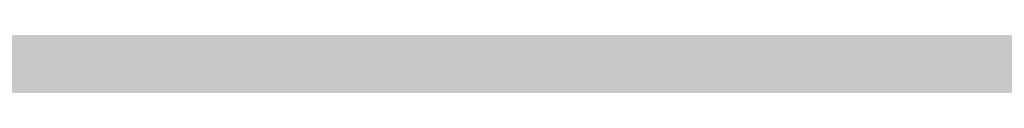
# Model space of a CAD drawing. Units: millimetres. Extents: x 0 to 2267, y 0 to 1823.
# Tile 54 of 256: x 1596.855 to 1600.369, y 1227.02 to 1227.171. Entities that reach past the tile are written whole.
import ezdxf

# ---------------------------------------------------------------- set-up
doc = ezdxf.new("R2010")
doc.units = ezdxf.units.MM
doc.header["$MEASUREMENT"] = 0
doc.layers.add('M-HATC', color=252, linetype='Continuous', lineweight=18)

msp = doc.modelspace()

# ---------------------------------------------------------------- hatches: boundary and pattern name
at = {"layer": 'M-HATC'}
h = msp.add_hatch(color=256, dxfattribs=at)
h.dxf.hatch_style = 1
h.paths.add_polyline_path([(2055.771, 1603.062), (1381.0868, 1603.062), (1381.0868, 1598.062), (2055.771, 1598.062)])
h.paths.add_polyline_path([(2055.771, 1598.062), (1381.0868, 1598.062), (1381.0868, 1593.062), (2055.771, 1593.062)])
h.paths.add_polyline_path([(2051.3074, 1536.7609), (1385.5504, 1536.7609), (1385.5504, 1526.7609), (1387.5504, 1526.7609), (1388.5366, 1525.0528), (1385.3319, 1521.2335), (1385.3319, 1521.2226), (2050.2542, 1522.7491), (2048.3212, 1525.0528), (2049.3074, 1526.7609), (2051.3074, 1526.7609)])
edge = h.paths.add_edge_path()
edge.add_arc((1847.5345, 1379.1492), 135, 222.603061, 222.890851, ccw=False)
edge.add_line((1748.1663, 1287.7656), (1683.0921, 1287.7656))
edge.add_arc((1583.7239, 1379.1492), 135, 317.109149, 317.396939, ccw=False)
edge.add_arc((1678.9686, 1290.6707), 5, 222.8909, 317.1091, ccw=False)
edge.add_arc((1774.2133, 1379.1492), 135, 222.603061, 222.890851, ccw=False)
edge.add_line((1674.8451, 1287.7656), (1609.7709, 1287.7656))
edge.add_arc((1510.4027, 1379.1492), 135, 317.109149, 317.396939, ccw=False)
edge.add_arc((1605.6474, 1290.6707), 5, 222.8909, 317.1091, ccw=False)
edge.add_arc((1700.8921, 1379.1492), 135, 222.603061, 222.890851, ccw=False)
edge.add_line((1601.5239, 1287.7656), (1536.4497, 1287.7656))
edge.add_arc((1437.0815, 1379.1492), 135, 317.109149, 317.396939, ccw=False)
edge.add_arc((1532.3262, 1290.6707), 5, 222.8909, 317.1091, ccw=False)
edge.add_arc((1627.5709, 1379.1492), 135, 222.603061, 222.890851, ccw=False)
edge.add_line((1528.2027, 1287.7656), (1505.9289, 1287.7656))
edge.add_spline(control_points=[(1505.9289, 1287.7656), (1504.2622, 1287.7656), (1504.2622, 1282.7656), (1505.9289, 1282.7656)], knot_values=[0, 0, 0, 0, 5, 5, 5, 5], degree=3, periodic=0)
edge.add_line((1505.9289, 1282.7656), (1930.9289, 1282.7656))
edge.add_spline(control_points=[(1930.9289, 1282.7656), (1932.5956, 1282.7656), (1932.5956, 1287.7656), (1930.9289, 1287.7656)], knot_values=[0, 0, 0, 0, 5, 5, 5, 5], degree=3, periodic=0)
edge.add_line((1930.9289, 1287.7656), (1903.0557, 1287.7656))
edge.add_arc((1803.6875, 1379.1492), 135, 317.109149, 317.396939, ccw=False)
edge.add_arc((1898.9322, 1290.6707), 5, 222.8909, 317.1091, ccw=False)
edge.add_arc((1994.1769, 1379.1492), 135, 222.603061, 222.890851, ccw=False)
edge.add_line((1894.8087, 1287.7656), (1829.7345, 1287.7656))
edge.add_arc((1730.3663, 1379.1492), 135, 317.109149, 317.396939, ccw=False)
edge.add_arc((1825.611, 1290.6707), 5, 222.8909, 317.1091, ccw=False)
edge.add_arc((1920.8557, 1379.1492), 135, 222.603061, 222.890851, ccw=False)
edge.add_line((1821.4875, 1287.7656), (1756.4133, 1287.7656))
edge.add_arc((1657.0451, 1379.1492), 135, 317.109149, 317.396939, ccw=False)
edge.add_arc((1752.2898, 1290.6707), 5, 222.8909, 317.1091, ccw=False)
edge = h.paths.add_edge_path()
edge.add_spline(control_points=[(1843.4289, 1227.2475), (1845.0956, 1227.2475), (1845.0956, 1232.2475), (1843.4289, 1232.2475)], knot_values=[0, 0, 0, 0, 5, 5, 5, 5], degree=3, periodic=0)
edge.add_line((1843.4289, 1232.2475), (1593.4289, 1232.2475))
edge.add_spline(control_points=[(1593.4289, 1232.2475), (1591.7622, 1232.2475), (1591.7622, 1227.2475), (1593.4289, 1227.2475)], knot_values=[0, 0, 0, 0, 5, 5, 5, 5], degree=3, periodic=0)
edge.add_line((1593.4289, 1227.2475), (1843.4289, 1227.2475))
h.paths.add_polyline_path([(1905.9289, 1127.4171), (1530.9289, 1127.4171, 0.414214), (1520.9289, 1117.4171), (1530.9289, 1117.4171), (1915.9289, 1117.4171, 0.414214)])
edge = h.paths.add_edge_path()
edge.add_arc((1397.0858, 1498.4078), 12.7299, 90.78215, 190.87871, ccw=False)
edge.add_line((1396.912, 1511.1365), (1428.0097, 1511.3488))
edge.add_line((1428.0097, 1511.3488), (1433.0097, 1511.3488))
edge.add_line((1433.0097, 1511.3488), (1434.439, 1511.3488))
edge.add_arc((1419.474, 1498.0804), 20, 41.561, 74.08211)
edge.add_line((1424.9592, 1517.3135), (1399.9351, 1517.2561))
edge.add_spline(control_points=[(1399.9307, 1517.2561), (1399.884, 1517.2131), (1399.8328, 1517.1689), (1399.7774, 1517.1236)], knot_values=[11.567499, 11.567499, 11.567499, 11.567499, 11.814249, 11.814249, 11.814249, 11.814249], degree=3, periodic=0)
edge.add_spline(control_points=[(1399.6328, 1517.0099), (1399.5831, 1516.9721), (1399.5307, 1516.9338), (1399.4759, 1516.8947)], knot_values=[11.167718, 11.167718, 11.167718, 11.167718, 11.365188, 11.365188, 11.365188, 11.365188], degree=3, periodic=0)
edge.add_spline(control_points=[(1399.3398, 1516.8001), (1399.1514, 1516.6719), (1398.9384, 1516.5377), (1398.704, 1516.3994)], knot_values=[10.376405, 10.376405, 10.376405, 10.376405, 11.00994, 11.00994, 11.00994, 11.00994], degree=3, periodic=0)
edge.add_spline(control_points=[(1398.6572, 1516.3719), (1398.5789, 1516.326), (1398.4983, 1516.2797), (1398.4155, 1516.2331)], knot_values=[10.125175, 10.125175, 10.125175, 10.125175, 10.334406, 10.334406, 10.334406, 10.334406], degree=3, periodic=0)
edge.add_spline(control_points=[(1398.2642, 1516.1487), (1398.196, 1516.1111), (1398.1263, 1516.0732), (1398.0555, 1516.0351)], knot_values=[9.832246, 9.832246, 9.832246, 9.832246, 9.999658, 9.999658, 9.999658, 9.999658], degree=3, periodic=0)
edge.add_spline(control_points=[(1397.9987, 1516.0048), (1397.7312, 1515.8621), (1397.446, 1515.7171), (1397.1466, 1515.5714)], knot_values=[9.161808, 9.161808, 9.161808, 9.161808, 9.787769, 9.787769, 9.787769, 9.787769], degree=3, periodic=0)
edge.add_spline(control_points=[(1397.1466, 1515.5714), (1396.8418, 1515.423), (1396.5222, 1515.274), (1396.1914, 1515.1262)], knot_values=[8.524455, 8.524455, 8.524455, 8.524455, 9.161808, 9.161808, 9.161808, 9.161808], degree=3, periodic=0)
edge.add_spline(control_points=[(1396.0777, 1515.0756), (1395.9854, 1515.0348), (1395.8922, 1514.994), (1395.7983, 1514.9534)], knot_values=[8.275193, 8.275193, 8.275193, 8.275193, 8.451726, 8.451726, 8.451726, 8.451726], degree=3, periodic=0)
edge.add_spline(control_points=[(1395.6018, 1514.8691), (1395.4997, 1514.8257), (1395.3968, 1514.7824), (1395.2932, 1514.7394)], knot_values=[7.962917, 7.962917, 7.962917, 7.962917, 8.152764, 8.152764, 8.152764, 8.152764], degree=3, periodic=0)
edge.add_spline(control_points=[(1395.2116, 1514.7057), (1394.8278, 1514.5475), (1394.4345, 1514.3929), (1394.0364, 1514.2442)], knot_values=[7.21254, 7.21254, 7.21254, 7.21254, 7.913148, 7.913148, 7.913148, 7.913148], degree=3, periodic=0)
edge.add_spline(control_points=[(1394.0364, 1514.2442), (1393.7076, 1514.1214), (1393.3754, 1514.0027), (1393.0427, 1513.8895)], knot_values=[6.633733, 6.633733, 6.633733, 6.633733, 7.21254, 7.21254, 7.21254, 7.21254], degree=3, periodic=0)
edge.add_spline(control_points=[(1392.8214, 1513.815), (1392.7198, 1513.7812), (1392.6181, 1513.7479), (1392.5166, 1513.7152)], knot_values=[6.328796, 6.328796, 6.328796, 6.328796, 6.505493, 6.505493, 6.505493, 6.505493], degree=3, periodic=0)
edge.add_spline(control_points=[(1392.5166, 1513.7152), (1392.3187, 1513.6515), (1392.1212, 1513.59), (1391.9244, 1513.531)], knot_values=[5.984605, 5.984605, 5.984605, 5.984605, 6.328796, 6.328796, 6.328796, 6.328796], degree=3, periodic=0)
edge.add_spline(control_points=[(1391.7915, 1513.4915), (1391.3122, 1513.3501), (1390.8384, 1513.2239), (1390.3784, 1513.1171)], knot_values=[5.066697, 5.066697, 5.066697, 5.066697, 5.907055, 5.907055, 5.907055, 5.907055], degree=3, periodic=0)
edge.add_spline(control_points=[(1390.3784, 1513.1171), (1390.1797, 1513.071), (1389.9836, 1513.0284), (1389.7907, 1512.9899)], knot_values=[4.70367, 4.70367, 4.70367, 4.70367, 5.066695, 5.066695, 5.066695, 5.066695], degree=3, periodic=0)
edge.add_spline(control_points=[(1389.422, 1512.9204), (1389.2459, 1512.8892), (1389.0729, 1512.8617), (1388.9036, 1512.8381)], knot_values=[4.130571, 4.130571, 4.130571, 4.130571, 4.469816, 4.469816, 4.469816, 4.469816], degree=3, periodic=0)
edge.add_spline(control_points=[(1388.9036, 1512.8381), (1388.591, 1512.7946), (1388.2911, 1512.7644), (1388.0071, 1512.7494)], knot_values=[3.504031, 3.504031, 3.504031, 3.504031, 4.130571, 4.130571, 4.130571, 4.130571], degree=3, periodic=0)
edge.add_spline(control_points=[(1387.9356, 1512.7459), (1387.8538, 1512.7423), (1387.7733, 1512.74), (1387.6944, 1512.739)], knot_values=[3.268866, 3.268866, 3.268866, 3.268866, 3.451164, 3.451164, 3.451164, 3.451164], degree=3, periodic=0)
edge.add_spline(control_points=[(1387.3351, 1512.7443), (1387.2076, 1512.7499), (1387.0847, 1512.7597), (1386.967, 1512.7739)], knot_values=[2.670686, 2.670686, 2.670686, 2.670686, 2.984, 2.984, 2.984, 2.984], degree=3, periodic=0)
edge.add_spline(control_points=[(1386.8327, 1512.7922), (1386.8209, 1512.7941), (1386.8092, 1512.7959), (1386.7975, 1512.7979)], knot_values=[2.516981, 2.516981, 2.516981, 2.516981, 2.549528, 2.549528, 2.549528, 2.549528], degree=3, periodic=0)
edge.add_spline(control_points=[(1386.4526, 1512.8735), (1386.4257, 1512.881), (1386.3993, 1512.889), (1386.3733, 1512.8972)], knot_values=[2.095869, 2.095869, 2.095869, 2.095869, 2.17941, 2.17941, 2.17941, 2.17941], degree=3, periodic=0)
edge.add_spline(control_points=[(1386.0691, 1513.0189), (1386.0634, 1513.0217), (1386.0577, 1513.0246), (1386.052, 1513.0275)], knot_values=[1.72453, 1.72453, 1.72453, 1.72453, 1.745933, 1.745933, 1.745933, 1.745933], degree=3, periodic=0)
edge.add_arc((1399.474, 1498.0804), 20, 131.82432, 180)
edge.add_arc((1630.3336, 1505.5484), 250.9708, 181.705176, 236.427975)
edge.add_arc((1605.3399, 1483.3044), 218.7822, 238.660829, 243.34961)
edge.add_arc((1647.0911, 1510.3592), 262.8986, 183.129836, 237.853442, ccw=False)
h.paths.add_polyline_path([(1406.5369, 1391.9644, 0.149382), (1491.5506, 1296.4418, -0.129517)], flags=17)
edge = h.paths.add_edge_path()
edge.add_arc((2037.3838, 1498.0804), 20, 0, 48.26587)
edge.add_spline(control_points=[(2050.6973, 1513.0052), (2050.6512, 1512.9847), (2050.6034, 1512.9655), (2050.5539, 1512.9477)], knot_values=[1.835652, 1.835652, 1.835652, 1.835652, 2.000781, 2.000781, 2.000781, 2.000781], degree=3, periodic=0)
edge.add_spline(control_points=[(2050.4616, 1512.9166), (2050.479, 1512.9221), (2050.4963, 1512.9277), (2050.5133, 1512.9335)], knot_values=[2.045477, 2.045477, 2.045477, 2.045477, 2.101389, 2.101389, 2.101389, 2.101389], degree=3, periodic=0)
edge.add_spline(control_points=[(2050.129, 1512.8342), (2050.1984, 1512.8473), (2050.2657, 1512.8623), (2050.3308, 1512.8792)], knot_values=[2.237629, 2.237629, 2.237629, 2.237629, 2.435841, 2.435841, 2.435841, 2.435841], degree=3, periodic=0)
edge.add_spline(control_points=[(2050.0946, 1512.8278), (2050.1061, 1512.8299), (2050.1176, 1512.832), (2050.129, 1512.8342)], knot_values=[2.435841, 2.435841, 2.435841, 2.435841, 2.468321, 2.468321, 2.468321, 2.468321], degree=3, periodic=0)
edge.add_spline(control_points=[(2049.7843, 1512.7851), (2049.8552, 1512.7922), (2049.9243, 1512.8008), (2049.9917, 1512.8109)], knot_values=[2.563852, 2.563852, 2.563852, 2.563852, 2.748541, 2.748541, 2.748541, 2.748541], degree=3, periodic=0)
edge.add_spline(control_points=[(2049.4052, 1512.7617), (2049.5364, 1512.7653), (2049.6629, 1512.773), (2049.7843, 1512.7851)], knot_values=[2.748541, 2.748541, 2.748541, 2.748541, 3.064882, 3.064882, 3.064882, 3.064882], degree=3, periodic=0)
edge.add_spline(control_points=[(2049.1698, 1512.7597), (2049.2336, 1512.7591), (2049.2965, 1512.7594), (2049.3584, 1512.7606)], knot_values=[3.102309, 3.102309, 3.102309, 3.102309, 3.2503, 3.2503, 3.2503, 3.2503], degree=3, periodic=0)
edge.add_spline(control_points=[(2048.8573, 1512.7691), (2048.9638, 1512.7638), (2049.068, 1512.7606), (2049.1698, 1512.7597)], knot_values=[3.2503, 3.2503, 3.2503, 3.2503, 3.486069, 3.486069, 3.486069, 3.486069], degree=3, periodic=0)
edge.add_spline(control_points=[(2048.6924, 1512.7789), (2048.3729, 1512.8009), (2048.0345, 1512.8411), (2047.6817, 1512.897)], knot_values=[3.606429, 3.606429, 3.606429, 3.606429, 4.2989, 4.2989, 4.2989, 4.2989], degree=3, periodic=0)
edge.add_spline(control_points=[(2047.6817, 1512.897), (2047.5458, 1512.9185), (2047.4077, 1512.9424), (2047.2678, 1512.9685)], knot_values=[4.2989, 4.2989, 4.2989, 4.2989, 4.565769, 4.565769, 4.565769, 4.565769], degree=3, periodic=0)
edge.add_spline(control_points=[(2047.2678, 1512.9685), (2047.1449, 1512.9914), (2047.0207, 1513.016), (2046.8951, 1513.0422)], knot_values=[4.565769, 4.565769, 4.565769, 4.565769, 4.799971, 4.799971, 4.799971, 4.799971], degree=3, periodic=0)
edge.add_spline(control_points=[(2046.8951, 1513.0422), (2046.5286, 1513.1188), (2046.1513, 1513.209), (2045.7676, 1513.3107)], knot_values=[4.799971, 4.799971, 4.799971, 4.799971, 5.483718, 5.483718, 5.483718, 5.483718], degree=3, periodic=0)
edge.add_spline(control_points=[(2045.7676, 1513.3107), (2045.3724, 1513.4154), (2044.9704, 1513.5322), (2044.5662, 1513.6588)], knot_values=[5.483718, 5.483718, 5.483718, 5.483718, 6.187866, 6.187866, 6.187866, 6.187866], degree=3, periodic=0)
edge.add_spline(control_points=[(2044.5662, 1513.6588), (2044.4149, 1513.7061), (2044.2633, 1513.7549), (2044.1116, 1513.8048)], knot_values=[6.187866, 6.187866, 6.187866, 6.187866, 6.451551, 6.451551, 6.451551, 6.451551], degree=3, periodic=0)
edge.add_spline(control_points=[(2044.1116, 1513.8048), (2043.9967, 1513.8427), (2043.8817, 1513.8813), (2043.7668, 1513.9205)], knot_values=[6.451551, 6.451551, 6.451551, 6.451551, 6.651434, 6.651434, 6.651434, 6.651434], degree=3, periodic=0)
edge.add_spline(control_points=[(2043.7668, 1513.9205), (2043.3716, 1514.0554), (2042.9774, 1514.1979), (2042.5886, 1514.3458)], knot_values=[6.651434, 6.651434, 6.651434, 6.651434, 7.338879, 7.338879, 7.338879, 7.338879], degree=3, periodic=0)
edge.add_spline(control_points=[(2042.5886, 1514.3458), (2042.1643, 1514.5071), (2041.7465, 1514.6749), (2041.3409, 1514.846)], knot_values=[7.338879, 7.338879, 7.338879, 7.338879, 8.089209, 8.089209, 8.089209, 8.089209], degree=3, periodic=0)
edge.add_spline(control_points=[(2041.3409, 1514.846), (2041.1028, 1514.9465), (2040.869, 1515.0481), (2040.6405, 1515.1502)], knot_values=[8.089209, 8.089209, 8.089209, 8.089209, 8.529587, 8.529587, 8.529587, 8.529587], degree=3, periodic=0)
edge.add_spline(control_points=[(2040.51, 1515.2089), (2040.0824, 1515.4022), (2039.6747, 1515.5971), (2039.295, 1515.7894)], knot_values=[8.613818, 8.613818, 8.613818, 8.613818, 9.44571, 9.44571, 9.44571, 9.44571], degree=3, periodic=0)
edge.add_spline(control_points=[(2039.295, 1515.7894), (2039.0618, 1515.9075), (2038.8391, 1516.0246), (2038.6288, 1516.1398)], knot_values=[9.44571, 9.44571, 9.44571, 9.44571, 9.956404, 9.956404, 9.956404, 9.956404], degree=3, periodic=0)
edge.add_spline(control_points=[(2038.6288, 1516.1398), (2038.5187, 1516.2001), (2038.4121, 1516.2598), (2038.309, 1516.3189)], knot_values=[9.956404, 9.956404, 9.956404, 9.956404, 10.223542, 10.223542, 10.223542, 10.223542], degree=3, periodic=0)
edge.add_spline(control_points=[(2038.309, 1516.3189), (2038.2138, 1516.3735), (2038.1216, 1516.4276), (2038.0328, 1516.481)], knot_values=[10.223542, 10.223542, 10.223542, 10.223542, 10.47051, 10.47051, 10.47051, 10.47051], degree=3, periodic=0)
edge.add_spline(control_points=[(2038.0328, 1516.481), (2037.7855, 1516.6296), (2037.5639, 1516.773), (2037.3722, 1516.909)], knot_values=[10.47051, 10.47051, 10.47051, 10.47051, 11.15767, 11.15767, 11.15767, 11.15767], degree=3, periodic=0)
edge.add_spline(control_points=[(2037.3722, 1516.909), (2037.2789, 1516.9752), (2037.1927, 1517.0396), (2037.1142, 1517.102)], knot_values=[11.15767, 11.15767, 11.15767, 11.15767, 11.49227, 11.49227, 11.49227, 11.49227], degree=3, periodic=0)
edge.add_spline(control_points=[(2036.8564, 1517.3259), (2036.9148, 1517.2692), (2036.9814, 1517.2103), (2037.0557, 1517.1492)], knot_values=[11.577341, 11.577341, 11.577341, 11.577341, 11.91035, 11.91035, 11.91035, 11.91035], degree=3, periodic=0)
edge.add_spline(control_points=[(2036.8074, 1517.3748), (2036.823, 1517.3587), (2036.8393, 1517.3424), (2036.8564, 1517.3259)], knot_values=[11.91035, 11.91035, 11.91035, 11.91035, 12.007402, 12.007402, 12.007402, 12.007402], degree=3, periodic=0)
edge.add_spline(control_points=[(2036.7017, 1517.494), (2036.7104, 1517.483), (2036.7196, 1517.4719), (2036.7291, 1517.4606)], knot_values=[12.184155, 12.184155, 12.184155, 12.184155, 12.255409, 12.255409, 12.255409, 12.255409], degree=3, periodic=0)
edge.add_spline(control_points=[(2036.6159, 1517.6205), (2036.62, 1517.613), (2036.6243, 1517.6055), (2036.6289, 1517.5979)], knot_values=[12.487913, 12.487913, 12.487913, 12.487913, 12.541035, 12.541035, 12.541035, 12.541035], degree=3, periodic=0)
edge.add_spline(control_points=[(2036.5635, 1517.786), (2036.5637, 1517.7794), (2036.5642, 1517.7726), (2036.565, 1517.7658)], knot_values=[12.911761, 12.911761, 12.911761, 12.911761, 12.968286, 12.968286, 12.968286, 12.968286], degree=3, periodic=0)
edge.add_spline(control_points=[(2036.6166, 1517.9304), (2036.6125, 1517.9259), (2036.6086, 1517.9212), (2036.6049, 1517.9165)], knot_values=[13.382527, 13.382527, 13.382527, 13.382527, 13.433791, 13.433791, 13.433791, 13.433791], degree=3, periodic=0)
edge.add_spline(control_points=[(2036.749, 1518.017), (2036.7361, 1518.0116), (2036.7239, 1518.006), (2036.7124, 1518.0002)], knot_values=[13.726299, 13.726299, 13.726299, 13.726299, 13.809928, 13.809928, 13.809928, 13.809928], degree=3, periodic=0)
edge.add_spline(control_points=[(2036.8604, 1518.0528), (2036.8386, 1518.0474), (2036.8181, 1518.0416), (2036.7988, 1518.0353)], knot_values=[13.910887, 13.910887, 13.910887, 13.910887, 14.02153, 14.02153, 14.02153, 14.02153], degree=3, periodic=0)
edge.add_line((2036.9639, 1518.0804), (2032.3838, 1518.0804))
edge.add_line((2032.3838, 1518.0804), (2027.3838, 1518.0804))
edge.add_line((2027.3838, 1518.0804), (2022.3838, 1518.0804))
edge.add_line((2022.3838, 1518.0804), (2017.3838, 1518.0804))
edge.add_arc((2017.3838, 1498.0804), 20, 90, 138.439)
edge.add_line((2002.4188, 1511.3488), (2003.8481, 1511.3488))
edge.add_line((2003.8481, 1511.3488), (2008.8481, 1511.3488))
edge.add_line((2008.8481, 1511.3488), (2039.772, 1511.1377))
edge.add_arc((2039.772, 1498.4078), 12.7299, -10.87871, 90, ccw=False)
edge.add_arc((1789.7668, 1510.3592), 262.8986, 302.146558, 356.870164, ccw=False)
edge.add_arc((1831.5179, 1483.3044), 218.7822, 296.65039, 301.339171)
edge.add_arc((1806.5242, 1505.5484), 250.9708, 303.572025, 358.294824)
h.paths.add_polyline_path([(2030.321, 1391.9644, -0.129517), (1945.3072, 1296.4418, 0.149382)], flags=17)
edge = h.paths.add_edge_path()
edge.add_spline(control_points=[(2037.2464, 1518.0821), (2037.2898, 1518.081), (2037.3355, 1518.0804), (2037.3838, 1518.0804)], knot_values=[0.000012, 0.000012, 0.000012, 0.000012, 0.144754, 0.144754, 0.144754, 0.144754], degree=3, periodic=0)
edge.add_line((2037.3357, 1518.0804), (2037.0096, 1518.0804))
edge.add_spline(control_points=[(2037.0096, 1518.0804), (2036.9822, 1518.0768), (2036.956, 1518.0727), (2036.9312, 1518.0681)], knot_values=[14.13465, 14.13465, 14.13465, 14.13465, 14.247197, 14.247197, 14.247197, 14.247197], degree=3, periodic=0)
edge.add_spline(control_points=[(2036.9312, 1518.0681), (2036.9276, 1518.0674), (2036.9241, 1518.0667), (2036.9205, 1518.0661)], knot_values=[14.118315, 14.118315, 14.118315, 14.118315, 14.13465, 14.13465, 14.13465, 14.13465], degree=3, periodic=0)
edge.add_spline(control_points=[(2036.9205, 1518.0661), (2036.9118, 1518.0644), (2036.9032, 1518.0626), (2036.8948, 1518.0608)], knot_values=[14.078086, 14.078086, 14.078086, 14.078086, 14.118315, 14.118315, 14.118315, 14.118315], degree=3, periodic=0)
edge.add_spline(control_points=[(2036.8948, 1518.0608), (2036.883, 1518.0583), (2036.8716, 1518.0556), (2036.8604, 1518.0528)], knot_values=[14.02153, 14.02153, 14.02153, 14.02153, 14.078086, 14.078086, 14.078086, 14.078086], degree=3, periodic=0)
edge.add_spline(control_points=[(2036.8604, 1518.0528), (2036.8386, 1518.0474), (2036.8181, 1518.0416), (2036.7988, 1518.0353)], knot_values=[13.910887, 13.910887, 13.910887, 13.910887, 14.02153, 14.02153, 14.02153, 14.02153], degree=3, periodic=0)
edge.add_spline(control_points=[(2036.7988, 1518.0353), (2036.7981, 1518.035), (2036.7974, 1518.0348), (2036.7967, 1518.0346)], knot_values=[13.906906, 13.906906, 13.906906, 13.906906, 13.910887, 13.910887, 13.910887, 13.910887], degree=3, periodic=0)
edge.add_spline(control_points=[(2036.7967, 1518.0346), (2036.7882, 1518.0318), (2036.7799, 1518.0289), (2036.7719, 1518.0259)], knot_values=[13.857826, 13.857826, 13.857826, 13.857826, 13.906906, 13.906906, 13.906906, 13.906906], degree=3, periodic=0)
edge.add_spline(control_points=[(2036.7719, 1518.0259), (2036.764, 1518.023), (2036.7564, 1518.02), (2036.749, 1518.017)], knot_values=[13.809928, 13.809928, 13.809928, 13.809928, 13.857826, 13.857826, 13.857826, 13.857826], degree=3, periodic=0)
edge.add_spline(control_points=[(2036.749, 1518.017), (2036.7361, 1518.0116), (2036.7239, 1518.006), (2036.7124, 1518.0002)], knot_values=[13.726299, 13.726299, 13.726299, 13.726299, 13.809928, 13.809928, 13.809928, 13.809928], degree=3, periodic=0)
edge.add_spline(control_points=[(2036.7124, 1518.0002), (2036.7121, 1518), (2036.7118, 1517.9999), (2036.7115, 1517.9997)], knot_values=[13.723993, 13.723993, 13.723993, 13.723993, 13.726299, 13.726299, 13.726299, 13.726299], degree=3, periodic=0)
edge.add_spline(control_points=[(2036.7115, 1517.9997), (2036.7063, 1517.9971), (2036.7013, 1517.9944), (2036.6965, 1517.9917)], knot_values=[13.686536, 13.686536, 13.686536, 13.686536, 13.723993, 13.723993, 13.723993, 13.723993], degree=3, periodic=0)
edge.add_spline(control_points=[(2036.6965, 1517.9917), (2036.6919, 1517.9891), (2036.6874, 1517.9865), (2036.6831, 1517.9839)], knot_values=[13.651251, 13.651251, 13.651251, 13.651251, 13.686536, 13.686536, 13.686536, 13.686536], degree=3, periodic=0)
edge.add_spline(control_points=[(2036.6831, 1517.9839), (2036.6764, 1517.9798), (2036.67, 1517.9757), (2036.6639, 1517.9714)], knot_values=[13.596804, 13.596804, 13.596804, 13.596804, 13.651251, 13.651251, 13.651251, 13.651251], degree=3, periodic=0)
edge.add_spline(control_points=[(2036.6639, 1517.9714), (2036.6636, 1517.9712), (2036.6633, 1517.9709), (2036.6629, 1517.9707)], knot_values=[13.593956, 13.593956, 13.593956, 13.593956, 13.596804, 13.596804, 13.596804, 13.596804], degree=3, periodic=0)
edge.add_spline(control_points=[(2036.6629, 1517.9707), (2036.6603, 1517.9689), (2036.6577, 1517.967), (2036.6552, 1517.9651)], knot_values=[13.570322, 13.570322, 13.570322, 13.570322, 13.593956, 13.593956, 13.593956, 13.593956], degree=3, periodic=0)
edge.add_spline(control_points=[(2036.6552, 1517.9651), (2036.6525, 1517.9631), (2036.6499, 1517.9611), (2036.6474, 1517.9591)], knot_values=[13.545477, 13.545477, 13.545477, 13.545477, 13.570322, 13.570322, 13.570322, 13.570322], degree=3, periodic=0)
edge.add_spline(control_points=[(2036.6474, 1517.9591), (2036.6472, 1517.9589), (2036.6471, 1517.9588), (2036.6469, 1517.9587)], knot_values=[13.543931, 13.543931, 13.543931, 13.543931, 13.545477, 13.545477, 13.545477, 13.545477], degree=3, periodic=0)
edge.add_spline(control_points=[(2036.6469, 1517.9587), (2036.6412, 1517.9541), (2036.6358, 1517.9494), (2036.6307, 1517.9447)], knot_values=[13.488237, 13.488237, 13.488237, 13.488237, 13.543931, 13.543931, 13.543931, 13.543931], degree=3, periodic=0)
edge.add_spline(control_points=[(2036.6307, 1517.9447), (2036.6282, 1517.9423), (2036.6257, 1517.9399), (2036.6233, 1517.9374)], knot_values=[13.460307, 13.460307, 13.460307, 13.460307, 13.488237, 13.488237, 13.488237, 13.488237], degree=3, periodic=0)
edge.add_spline(control_points=[(2036.6233, 1517.9374), (2036.6215, 1517.9356), (2036.6198, 1517.9338), (2036.6181, 1517.932)], knot_values=[13.439712, 13.439712, 13.439712, 13.439712, 13.460307, 13.460307, 13.460307, 13.460307], degree=3, periodic=0)
edge.add_spline(control_points=[(2036.6181, 1517.932), (2036.6176, 1517.9315), (2036.6171, 1517.9309), (2036.6166, 1517.9304)], knot_values=[13.433791, 13.433791, 13.433791, 13.433791, 13.439712, 13.439712, 13.439712, 13.439712], degree=3, periodic=0)
edge.add_spline(control_points=[(2036.6166, 1517.9304), (2036.6125, 1517.9259), (2036.6086, 1517.9212), (2036.6049, 1517.9165)], knot_values=[13.382527, 13.382527, 13.382527, 13.382527, 13.433791, 13.433791, 13.433791, 13.433791], degree=3, periodic=0)
edge.add_spline(control_points=[(2036.6049, 1517.9165), (2036.6026, 1517.9135), (2036.6004, 1517.9104), (2036.5982, 1517.9074)], knot_values=[13.350017, 13.350017, 13.350017, 13.350017, 13.382527, 13.382527, 13.382527, 13.382527], degree=3, periodic=0)
edge.add_spline(control_points=[(2036.5982, 1517.9074), (2036.5972, 1517.9059), (2036.5962, 1517.9043), (2036.5952, 1517.9028)], knot_values=[13.333922, 13.333922, 13.333922, 13.333922, 13.350017, 13.350017, 13.350017, 13.350017], degree=3, periodic=0)
edge.add_spline(control_points=[(2036.5952, 1517.9028), (2036.5945, 1517.9018), (2036.5939, 1517.9009), (2036.5933, 1517.8999)], knot_values=[13.323828, 13.323828, 13.323828, 13.323828, 13.333922, 13.333922, 13.333922, 13.333922], degree=3, periodic=0)
edge.add_spline(control_points=[(2036.5933, 1517.8999), (2036.5905, 1517.8955), (2036.5879, 1517.8909), (2036.5855, 1517.8864)], knot_values=[13.277545, 13.277545, 13.277545, 13.277545, 13.323828, 13.323828, 13.323828, 13.323828], degree=3, periodic=0)
edge.add_spline(control_points=[(2036.5855, 1517.8864), (2036.5836, 1517.8827), (2036.5817, 1517.8789), (2036.5801, 1517.8751)], knot_values=[13.240119, 13.240119, 13.240119, 13.240119, 13.277545, 13.277545, 13.277545, 13.277545], degree=3, periodic=0)
edge.add_spline(control_points=[(2036.5801, 1517.8751), (2036.5795, 1517.8739), (2036.579, 1517.8727), (2036.5785, 1517.8715)], knot_values=[13.228211, 13.228211, 13.228211, 13.228211, 13.240119, 13.240119, 13.240119, 13.240119], degree=3, periodic=0)
edge.add_spline(control_points=[(2036.5785, 1517.8715), (2036.578, 1517.8702), (2036.5774, 1517.869), (2036.5769, 1517.8677)], knot_values=[13.215717, 13.215717, 13.215717, 13.215717, 13.228211, 13.228211, 13.228211, 13.228211], degree=3, periodic=0)
edge.add_spline(control_points=[(2036.5769, 1517.8677), (2036.5755, 1517.864), (2036.5741, 1517.8603), (2036.5729, 1517.8565)], knot_values=[13.179847, 13.179847, 13.179847, 13.179847, 13.215717, 13.215717, 13.215717, 13.215717], degree=3, periodic=0)
edge.add_spline(control_points=[(2036.5729, 1517.8565), (2036.5713, 1517.8515), (2036.5699, 1517.8464), (2036.5687, 1517.8413)], knot_values=[13.132017, 13.132017, 13.132017, 13.132017, 13.179847, 13.179847, 13.179847, 13.179847], degree=3, periodic=0)
edge.add_spline(control_points=[(2036.5687, 1517.8413), (2036.5684, 1517.8402), (2036.5682, 1517.8392), (2036.568, 1517.8382)], knot_values=[13.122482, 13.122482, 13.122482, 13.122482, 13.132017, 13.132017, 13.132017, 13.132017], degree=3, periodic=0)
edge.add_spline(control_points=[(2036.568, 1517.8382), (2036.5676, 1517.8363), (2036.5672, 1517.8345), (2036.5669, 1517.8327)], knot_values=[13.105592, 13.105592, 13.105592, 13.105592, 13.122482, 13.122482, 13.122482, 13.122482], degree=3, periodic=0)
edge.add_spline(control_points=[(2036.5669, 1517.8327), (2036.5662, 1517.8292), (2036.5657, 1517.8257), (2036.5652, 1517.8222)], knot_values=[13.074063, 13.074063, 13.074063, 13.074063, 13.105592, 13.105592, 13.105592, 13.105592], degree=3, periodic=0)
edge.add_spline(control_points=[(2036.5652, 1517.8222), (2036.5652, 1517.8222), (2036.5652, 1517.8222), (2036.5652, 1517.8222)], knot_values=[13.074043, 13.074043, 13.074043, 13.074043, 13.074063, 13.074063, 13.074063, 13.074063], degree=3, periodic=0)
edge.add_spline(control_points=[(2036.5652, 1517.8222), (2036.5644, 1517.8164), (2036.5639, 1517.8106), (2036.5636, 1517.8046)], knot_values=[13.021884, 13.021884, 13.021884, 13.021884, 13.074043, 13.074043, 13.074043, 13.074043], degree=3, periodic=0)
edge.add_spline(control_points=[(2036.5636, 1517.8046), (2036.5636, 1517.804), (2036.5636, 1517.8034), (2036.5635, 1517.8028)], knot_values=[13.01674, 13.01674, 13.01674, 13.01674, 13.021884, 13.021884, 13.021884, 13.021884], degree=3, periodic=0)
edge.add_spline(control_points=[(2036.5635, 1517.8028), (2036.5634, 1517.8005), (2036.5634, 1517.7982), (2036.5634, 1517.7958)], knot_values=[12.996438, 12.996438, 12.996438, 12.996438, 13.01674, 13.01674, 13.01674, 13.01674], degree=3, periodic=0)
edge.add_spline(control_points=[(2036.5634, 1517.7958), (2036.5633, 1517.7926), (2036.5634, 1517.7893), (2036.5635, 1517.786)], knot_values=[12.968286, 12.968286, 12.968286, 12.968286, 12.996438, 12.996438, 12.996438, 12.996438], degree=3, periodic=0)
edge.add_spline(control_points=[(2036.5635, 1517.786), (2036.5637, 1517.7794), (2036.5642, 1517.7726), (2036.565, 1517.7658)], knot_values=[12.911761, 12.911761, 12.911761, 12.911761, 12.968286, 12.968286, 12.968286, 12.968286], degree=3, periodic=0)
edge.add_spline(control_points=[(2036.565, 1517.7658), (2036.565, 1517.7657), (2036.565, 1517.7656), (2036.565, 1517.7656)], knot_values=[12.911017, 12.911017, 12.911017, 12.911017, 12.911761, 12.911761, 12.911761, 12.911761], degree=3, periodic=0)
edge.add_spline(control_points=[(2036.565, 1517.7656), (2036.5654, 1517.7625), (2036.5658, 1517.7593), (2036.5663, 1517.7562)], knot_values=[12.88528, 12.88528, 12.88528, 12.88528, 12.911017, 12.911017, 12.911017, 12.911017], degree=3, periodic=0)
edge.add_spline(control_points=[(2036.5663, 1517.7562), (2036.5667, 1517.7534), (2036.5672, 1517.7506), (2036.5677, 1517.7478)], knot_values=[12.862519, 12.862519, 12.862519, 12.862519, 12.88528, 12.88528, 12.88528, 12.88528], degree=3, periodic=0)
edge.add_spline(control_points=[(2036.5677, 1517.7478), (2036.5678, 1517.7474), (2036.5679, 1517.7469), (2036.568, 1517.7465)], knot_values=[12.858885, 12.858885, 12.858885, 12.858885, 12.862519, 12.862519, 12.862519, 12.862519], degree=3, periodic=0)
edge.add_spline(control_points=[(2036.568, 1517.7465), (2036.5692, 1517.7399), (2036.5707, 1517.7332), (2036.5724, 1517.7264)], knot_values=[12.8053, 12.8053, 12.8053, 12.8053, 12.858885, 12.858885, 12.858885, 12.858885], degree=3, periodic=0)
edge.add_spline(control_points=[(2036.5724, 1517.7264), (2036.5734, 1517.7226), (2036.5745, 1517.7187), (2036.5756, 1517.7149)], knot_values=[12.775176, 12.775176, 12.775176, 12.775176, 12.8053, 12.8053, 12.8053, 12.8053], degree=3, periodic=0)
edge.add_spline(control_points=[(2036.5756, 1517.7149), (2036.5763, 1517.7125), (2036.577, 1517.7102), (2036.5778, 1517.7078)], knot_values=[12.756759, 12.756759, 12.756759, 12.756759, 12.775176, 12.775176, 12.775176, 12.775176], degree=3, periodic=0)
edge.add_spline(control_points=[(2036.5778, 1517.7078), (2036.5781, 1517.7067), (2036.5784, 1517.7057), (2036.5787, 1517.7047)], knot_values=[12.748742, 12.748742, 12.748742, 12.748742, 12.756759, 12.756759, 12.756759, 12.756759], degree=3, periodic=0)
edge.add_spline(control_points=[(2036.5787, 1517.7047), (2036.5808, 1517.6983), (2036.5831, 1517.6919), (2036.5856, 1517.6854)], knot_values=[12.69959, 12.69959, 12.69959, 12.69959, 12.748742, 12.748742, 12.748742, 12.748742], degree=3, periodic=0)
edge.add_spline(control_points=[(2036.5856, 1517.6854), (2036.5876, 1517.68), (2036.5898, 1517.6746), (2036.5921, 1517.6692)], knot_values=[12.659038, 12.659038, 12.659038, 12.659038, 12.69959, 12.69959, 12.69959, 12.69959], degree=3, periodic=0)
edge.add_spline(control_points=[(2036.5921, 1517.6692), (2036.594, 1517.6648), (2036.5959, 1517.6605), (2036.5979, 1517.6561)], knot_values=[12.626806, 12.626806, 12.626806, 12.626806, 12.659038, 12.659038, 12.659038, 12.659038], degree=3, periodic=0)
edge.add_spline(control_points=[(2036.5979, 1517.6561), (2036.5984, 1517.6551), (2036.5989, 1517.6541), (2036.5993, 1517.6531)], knot_values=[12.619394, 12.619394, 12.619394, 12.619394, 12.626806, 12.626806, 12.626806, 12.626806], degree=3, periodic=0)
edge.add_spline(control_points=[(2036.5993, 1517.6531), (2036.6043, 1517.6424), (2036.6099, 1517.6315), (2036.6159, 1517.6205)], knot_values=[12.541039, 12.541039, 12.541039, 12.541039, 12.619394, 12.619394, 12.619394, 12.619394], degree=3, periodic=0)
edge.add_spline(control_points=[(2036.6159, 1517.6205), (2036.6159, 1517.6205), (2036.6159, 1517.6205), (2036.6159, 1517.6205)], knot_values=[12.541035, 12.541035, 12.541035, 12.541035, 12.541039, 12.541039, 12.541039, 12.541039], degree=3, periodic=0)
edge.add_spline(control_points=[(2036.6159, 1517.6205), (2036.62, 1517.613), (2036.6243, 1517.6055), (2036.6289, 1517.5979)], knot_values=[12.487913, 12.487913, 12.487913, 12.487913, 12.541035, 12.541035, 12.541035, 12.541035], degree=3, periodic=0)
edge.add_spline(control_points=[(2036.6289, 1517.5979), (2036.6326, 1517.5916), (2036.6365, 1517.5853), (2036.6406, 1517.5789)], knot_values=[12.443982, 12.443982, 12.443982, 12.443982, 12.487913, 12.487913, 12.487913, 12.487913], degree=3, periodic=0)
edge.add_spline(control_points=[(2036.6406, 1517.5789), (2036.6414, 1517.5776), (2036.6423, 1517.5763), (2036.6431, 1517.5749)], knot_values=[12.434996, 12.434996, 12.434996, 12.434996, 12.443982, 12.443982, 12.443982, 12.443982], degree=3, periodic=0)
edge.add_spline(control_points=[(2036.6431, 1517.5749), (2036.6531, 1517.5596), (2036.6639, 1517.5439), (2036.6756, 1517.528)], knot_values=[12.329647, 12.329647, 12.329647, 12.329647, 12.434996, 12.434996, 12.434996, 12.434996], degree=3, periodic=0)
edge.add_spline(control_points=[(2036.6756, 1517.528), (2036.6839, 1517.5168), (2036.6925, 1517.5055), (2036.7017, 1517.494)], knot_values=[12.255409, 12.255409, 12.255409, 12.255409, 12.329647, 12.329647, 12.329647, 12.329647], degree=3, periodic=0)
edge.add_spline(control_points=[(2036.7017, 1517.494), (2036.7104, 1517.483), (2036.7196, 1517.4719), (2036.7291, 1517.4606)], knot_values=[12.184155, 12.184155, 12.184155, 12.184155, 12.255409, 12.255409, 12.255409, 12.255409], degree=3, periodic=0)
edge.add_spline(control_points=[(2036.7291, 1517.4606), (2036.7436, 1517.4435), (2036.759, 1517.4262), (2036.7753, 1517.4085)], knot_values=[12.075961, 12.075961, 12.075961, 12.075961, 12.184155, 12.184155, 12.184155, 12.184155], degree=3, periodic=0)
edge.add_spline(control_points=[(2036.7753, 1517.4085), (2036.7763, 1517.4075), (2036.7773, 1517.4064), (2036.7783, 1517.4054)], knot_values=[12.069502, 12.069502, 12.069502, 12.069502, 12.075961, 12.075961, 12.075961, 12.075961], degree=3, periodic=0)
edge.add_spline(control_points=[(2036.7783, 1517.4054), (2036.7877, 1517.3953), (2036.7974, 1517.385), (2036.8074, 1517.3748)], knot_values=[12.007402, 12.007402, 12.007402, 12.007402, 12.069502, 12.069502, 12.069502, 12.069502], degree=3, periodic=0)
edge.add_spline(control_points=[(2036.8074, 1517.3748), (2036.823, 1517.3587), (2036.8393, 1517.3424), (2036.8564, 1517.3259)], knot_values=[11.91035, 11.91035, 11.91035, 11.91035, 12.007402, 12.007402, 12.007402, 12.007402], degree=3, periodic=0)
edge.add_spline(control_points=[(2036.8564, 1517.3259), (2036.9148, 1517.2692), (2036.9814, 1517.2103), (2037.0557, 1517.1492)], knot_values=[11.577341, 11.577341, 11.577341, 11.577341, 11.91035, 11.91035, 11.91035, 11.91035], degree=3, periodic=0)
edge.add_spline(control_points=[(2037.0557, 1517.1492), (2037.0747, 1517.1336), (2037.0942, 1517.1179), (2037.1142, 1517.102)], knot_values=[11.49227, 11.49227, 11.49227, 11.49227, 11.577341, 11.577341, 11.577341, 11.577341], degree=3, periodic=0)
edge.add_spline(control_points=[(2037.1142, 1517.102), (2037.1927, 1517.0396), (2037.2789, 1516.9752), (2037.3722, 1516.909)], knot_values=[11.15767, 11.15767, 11.15767, 11.15767, 11.49227, 11.49227, 11.49227, 11.49227], degree=3, periodic=0)
edge.add_spline(control_points=[(2037.3722, 1516.909), (2037.5639, 1516.773), (2037.7855, 1516.6296), (2038.0328, 1516.481)], knot_values=[10.47051, 10.47051, 10.47051, 10.47051, 11.15767, 11.15767, 11.15767, 11.15767], degree=3, periodic=0)
edge.add_spline(control_points=[(2038.0328, 1516.481), (2038.1216, 1516.4276), (2038.2138, 1516.3735), (2038.309, 1516.3189)], knot_values=[10.223542, 10.223542, 10.223542, 10.223542, 10.47051, 10.47051, 10.47051, 10.47051], degree=3, periodic=0)
edge.add_spline(control_points=[(2038.309, 1516.3189), (2038.4121, 1516.2598), (2038.5187, 1516.2001), (2038.6288, 1516.1398)], knot_values=[9.956404, 9.956404, 9.956404, 9.956404, 10.223542, 10.223542, 10.223542, 10.223542], degree=3, periodic=0)
edge.add_spline(control_points=[(2038.6288, 1516.1398), (2038.8391, 1516.0246), (2039.0618, 1515.9075), (2039.295, 1515.7894)], knot_values=[9.44571, 9.44571, 9.44571, 9.44571, 9.956404, 9.956404, 9.956404, 9.956404], degree=3, periodic=0)
edge.add_spline(control_points=[(2039.295, 1515.7894), (2039.6747, 1515.5971), (2040.0824, 1515.4022), (2040.51, 1515.2089)], knot_values=[8.613818, 8.613818, 8.613818, 8.613818, 9.44571, 9.44571, 9.44571, 9.44571], degree=3, periodic=0)
edge.add_spline(control_points=[(2040.51, 1515.2089), (2040.5533, 1515.1893), (2040.5968, 1515.1697), (2040.6405, 1515.1502)], knot_values=[8.529587, 8.529587, 8.529587, 8.529587, 8.613818, 8.613818, 8.613818, 8.613818], degree=3, periodic=0)
edge.add_spline(control_points=[(2040.6405, 1515.1502), (2040.869, 1515.0481), (2041.1028, 1514.9465), (2041.3409, 1514.846)], knot_values=[8.089209, 8.089209, 8.089209, 8.089209, 8.529587, 8.529587, 8.529587, 8.529587], degree=3, periodic=0)
edge.add_spline(control_points=[(2041.3409, 1514.846), (2041.7465, 1514.6749), (2042.1643, 1514.5071), (2042.5886, 1514.3458)], knot_values=[7.338879, 7.338879, 7.338879, 7.338879, 8.089209, 8.089209, 8.089209, 8.089209], degree=3, periodic=0)
edge.add_spline(control_points=[(2042.5886, 1514.3458), (2042.9774, 1514.1979), (2043.3716, 1514.0554), (2043.7668, 1513.9205)], knot_values=[6.651434, 6.651434, 6.651434, 6.651434, 7.338879, 7.338879, 7.338879, 7.338879], degree=3, periodic=0)
edge.add_spline(control_points=[(2043.7668, 1513.9205), (2043.8817, 1513.8813), (2043.9967, 1513.8427), (2044.1116, 1513.8048)], knot_values=[6.451551, 6.451551, 6.451551, 6.451551, 6.651434, 6.651434, 6.651434, 6.651434], degree=3, periodic=0)
edge.add_spline(control_points=[(2044.1116, 1513.8048), (2044.2633, 1513.7549), (2044.4149, 1513.7061), (2044.5662, 1513.6588)], knot_values=[6.187866, 6.187866, 6.187866, 6.187866, 6.451551, 6.451551, 6.451551, 6.451551], degree=3, periodic=0)
edge.add_spline(control_points=[(2044.5662, 1513.6588), (2044.9704, 1513.5322), (2045.3724, 1513.4154), (2045.7676, 1513.3107)], knot_values=[5.483718, 5.483718, 5.483718, 5.483718, 6.187866, 6.187866, 6.187866, 6.187866], degree=3, periodic=0)
edge.add_spline(control_points=[(2045.7676, 1513.3107), (2046.1513, 1513.209), (2046.5286, 1513.1188), (2046.8951, 1513.0422)], knot_values=[4.799971, 4.799971, 4.799971, 4.799971, 5.483718, 5.483718, 5.483718, 5.483718], degree=3, periodic=0)
edge.add_spline(control_points=[(2046.8951, 1513.0422), (2047.0207, 1513.016), (2047.1449, 1512.9914), (2047.2678, 1512.9685)], knot_values=[4.565769, 4.565769, 4.565769, 4.565769, 4.799971, 4.799971, 4.799971, 4.799971], degree=3, periodic=0)
edge.add_spline(control_points=[(2047.2678, 1512.9685), (2047.4077, 1512.9424), (2047.5458, 1512.9185), (2047.6817, 1512.897)], knot_values=[4.2989, 4.2989, 4.2989, 4.2989, 4.565769, 4.565769, 4.565769, 4.565769], degree=3, periodic=0)
edge.add_spline(control_points=[(2047.6817, 1512.897), (2048.0345, 1512.8411), (2048.3729, 1512.8009), (2048.6924, 1512.7789)], knot_values=[3.606429, 3.606429, 3.606429, 3.606429, 4.2989, 4.2989, 4.2989, 4.2989], degree=3, periodic=0)
edge.add_spline(control_points=[(2048.6924, 1512.7789), (2048.7479, 1512.7751), (2048.8029, 1512.7718), (2048.8573, 1512.7691)], knot_values=[3.486069, 3.486069, 3.486069, 3.486069, 3.606429, 3.606429, 3.606429, 3.606429], degree=3, periodic=0)
edge.add_spline(control_points=[(2048.8573, 1512.7691), (2048.9638, 1512.7638), (2049.068, 1512.7606), (2049.1698, 1512.7597)], knot_values=[3.2503, 3.2503, 3.2503, 3.2503, 3.486069, 3.486069, 3.486069, 3.486069], degree=3, periodic=0)
edge.add_spline(control_points=[(2049.1698, 1512.7597), (2049.2336, 1512.7591), (2049.2965, 1512.7594), (2049.3584, 1512.7606)], knot_values=[3.102309, 3.102309, 3.102309, 3.102309, 3.2503, 3.2503, 3.2503, 3.2503], degree=3, periodic=0)
edge.add_spline(control_points=[(2049.3584, 1512.7606), (2049.3741, 1512.7609), (2049.3897, 1512.7613), (2049.4052, 1512.7617)], knot_values=[3.064882, 3.064882, 3.064882, 3.064882, 3.102309, 3.102309, 3.102309, 3.102309], degree=3, periodic=0)
edge.add_spline(control_points=[(2049.4052, 1512.7617), (2049.5364, 1512.7653), (2049.6629, 1512.773), (2049.7843, 1512.7851)], knot_values=[2.748541, 2.748541, 2.748541, 2.748541, 3.064882, 3.064882, 3.064882, 3.064882], degree=3, periodic=0)
edge.add_spline(control_points=[(2049.7843, 1512.7851), (2049.8552, 1512.7922), (2049.9243, 1512.8008), (2049.9917, 1512.8109)], knot_values=[2.563852, 2.563852, 2.563852, 2.563852, 2.748541, 2.748541, 2.748541, 2.748541], degree=3, periodic=0)
edge.add_spline(control_points=[(2049.9917, 1512.8109), (2050.0265, 1512.8161), (2050.0608, 1512.8218), (2050.0946, 1512.8278)], knot_values=[2.468321, 2.468321, 2.468321, 2.468321, 2.563852, 2.563852, 2.563852, 2.563852], degree=3, periodic=0)
edge.add_spline(control_points=[(2050.0946, 1512.8278), (2050.1061, 1512.8299), (2050.1176, 1512.832), (2050.129, 1512.8342)], knot_values=[2.435841, 2.435841, 2.435841, 2.435841, 2.468321, 2.468321, 2.468321, 2.468321], degree=3, periodic=0)
edge.add_spline(control_points=[(2050.129, 1512.8342), (2050.1984, 1512.8473), (2050.2657, 1512.8623), (2050.3308, 1512.8792)], knot_values=[2.237629, 2.237629, 2.237629, 2.237629, 2.435841, 2.435841, 2.435841, 2.435841], degree=3, periodic=0)
edge.add_spline(control_points=[(2050.3308, 1512.8792), (2050.3754, 1512.8908), (2050.4191, 1512.9032), (2050.4616, 1512.9166)], knot_values=[2.101389, 2.101389, 2.101389, 2.101389, 2.237629, 2.237629, 2.237629, 2.237629], degree=3, periodic=0)
edge.add_spline(control_points=[(2050.4616, 1512.9166), (2050.479, 1512.9221), (2050.4963, 1512.9277), (2050.5133, 1512.9335)], knot_values=[2.045477, 2.045477, 2.045477, 2.045477, 2.101389, 2.101389, 2.101389, 2.101389], degree=3, periodic=0)
edge.add_spline(control_points=[(2050.5133, 1512.9335), (2050.527, 1512.9382), (2050.5405, 1512.9429), (2050.5539, 1512.9477)], knot_values=[2.000781, 2.000781, 2.000781, 2.000781, 2.045477, 2.045477, 2.045477, 2.045477], degree=3, periodic=0)
edge.add_spline(control_points=[(2050.5539, 1512.9477), (2050.6034, 1512.9655), (2050.6512, 1512.9847), (2050.6973, 1513.0052)], knot_values=[1.835652, 1.835652, 1.835652, 1.835652, 2.000781, 2.000781, 2.000781, 2.000781], degree=3, periodic=0)
edge.add_arc((2037.3838, 1498.0804), 20, 48.26587, 90.12993)
edge = h.paths.add_edge_path(flags=16)
edge.add_spline(control_points=[(1386.1389, 1512.9859), (1388.92, 1511.7395), (1398.0387, 1515.5187), (1399.9307, 1517.2561)], knot_values=[1.831046, 1.831046, 1.831046, 1.831046, 11.814249, 11.814249, 11.814249, 11.814249], degree=3, periodic=0)
edge.add_line((1399.9307, 1517.2561), (1393.7435, 1517.2419))
edge.add_arc((1399.474, 1498.0804), 20, 106.6501, 131.8173)
h = msp.add_hatch(color=256, dxfattribs=at)
h.dxf.hatch_style = 1
h.paths.add_polyline_path([(2042.8886, 1580.1796), (2055.771, 1593.062), (1381.0868, 1593.062), (1393.9692, 1580.1796), (1374.086, 1560.2964), (2062.7718, 1560.2964)])
h.paths.add_polyline_path([(1843.4289, 1201.3297), (1843.4289, 1227.2475), (1593.4289, 1227.2475), (1593.4289, 1201.3297, -0.228274), (1574.5989, 1162.2346), (1530.9289, 1127.4171), (1905.9289, 1127.4171), (1862.2589, 1162.2346, -0.228274)])

doc.saveas('drawing.dxf')
